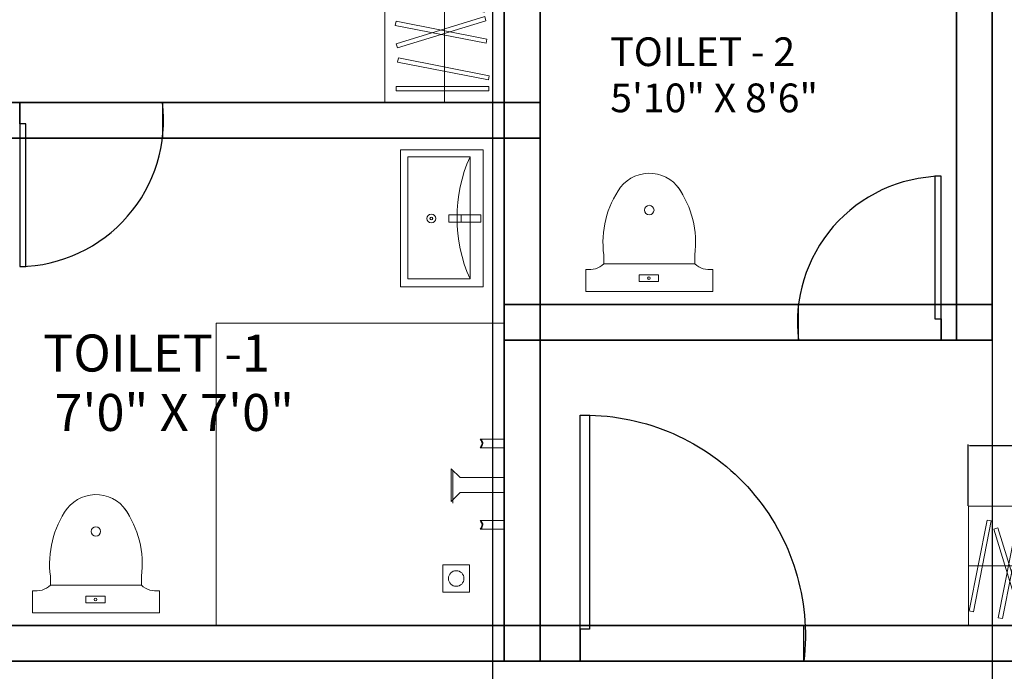
# Model space of a CAD drawing. Units: inches. Extents: x -61 to 1599, y -1316 to 257.
# Tile 67 of 204: x 240 to 406, y -790 to -680. Entities that reach past the tile are written whole.
import ezdxf

# ---------------------------------------------------------------- set-up
doc = ezdxf.new("R2010")
doc.units = ezdxf.units.IN
doc.header["$MEASUREMENT"] = 0
doc.linetypes.add('ACAD_ISO02W100', pattern=[15, 12, -3])
for name, color, linetype, lineweight in [('A-ANNO-DIMS', 2, 'Continuous', 18), ('A-AREA-IDEN', 1, 'Continuous', 18), ('A-FLOR-CASE', 8, 'Continuous', 18), ('A-FLOR-FIXT', 8, 'Continuous', 18), ('A-WALL-JAMB', 4, 'ACAD_ISO02W100', 25), ('DOORS', 2, 'Continuous', 25), ('WALLS', 4, 'Continuous', 35)]:
    doc.layers.add(name, color=color, linetype=linetype, lineweight=lineweight)
doc.styles.get("Standard").update_dxf_attribs({"font": 'arial.ttf'})
doc.dimstyles.get("Standard").update_dxf_attribs({"dimtxt": 0.18, "dimasz": 0.18, "dimexe": 0.18, "dimexo": 0.0625, "dimgap": 0.09, "dimtad": 0, "dimtih": 1, "dimtoh": 1, "dimdec": 0, "dimzin": 0, "dimdsep": 46, "dimlunit": 3, "dimtxsty": 'Standard', "dimcen": 0.09, "dimadec": 0, "dimazin": 0, "dimtfac": 1, "dimtdec": 0, "dimtofl": 0, "dimtmove": 0, "dimatfit": 3, "dimfxl": 1, "dimtolj": 1, "dimtzin": 0, "dimarcsym": 0})

# ---------------------------------------------------------------- blocks, each defined once
blk = doc.blocks.new('DOOR-SWING-24')
blk.add_line((0, 0), (0, 3.6))
blk.add_lwpolyline([(0, 0), (0, -24), (1.05, -24), (1.05, 0)], close=True)
blk.add_arc((-0.44, 0.62), 24.62, 271.0259, 6.9559)
blk = doc.blocks.new('DOOR-SWING-36')
blk.add_line((0, 0), (0, -5.4))
blk.add_lwpolyline([(0, 0), (0, 36), (-1.57, 36), (-1.57, 0)], close=True)
blk.add_arc((-0.74, -1.08), 37.09, 91.2913, 186.6905)
blk = doc.blocks.new('WC-FLOOR-MOUNT')
for p, q in [((3.02, 4.69), (3.02, 6.17)), ((18.31, 4.69), (18.31, 6.17)), ((0, 0), (0, 3.75)), ((3.02, 4.69), (18.31, 4.69)), ((21.33, 0), (21.33, 3.75)), ((0, 0), (21.33, 0))]:
    blk.add_line(p, q)
blk.add_lwpolyline([(12.24, 1.73), (8.96, 1.73), (8.96, 2.81), (12.24, 2.81)], close=True)
for centre, radius in [((10.67, 13.73), 0.792), ((10.6, 2.27), 0.208)]:
    blk.add_circle(centre, radius)
for centre, radius, start, end in [((10.67, 13.73), 6.18, 27.6844, 141.4697), ((19.05, 8.26), 16.17, 144.824, 187.4232), ((2.28, 8.26), 16.17, 352.5768, 35.176), ((0.56, 7.25), 3.55, 260.8586, 313.6993), ((20.77, 7.25), 3.55, 226.3007, 279.1414)]:
    blk.add_arc(centre, radius, start, end)
blk = doc.blocks.new('LAVATORY-WALL')
blk.add_line((10.19, 12.11), (10.19, 10.88))
for points in [[(13.87, 0), (0, 0), (0, 23.07), (13.87, 23.07)], [(13.87, 0), (0, 0), (0, 23.07), (13.87, 23.07)], [(1.2, 1.34), (1.2, 21.88), (11.67, 21.88), (11.67, 1.34)], [(8.09, 10.88), (8.09, 12.11), (13.47, 12.11), (13.47, 10.88)]]:
    blk.add_lwpolyline(points, close=True)
for radius in [0.74, 0.233]:
    blk.add_circle((5.16, 11.5), radius)
blk.add_arc((34.73, 11.61), 25.25, 155.9939, 204.0061)
blk = doc.blocks.new('SHOWER-FITTINGS')
for p, q in [((10.35, 25.72), (6.31, 25.72)), ((10.35, 24.3), (6.31, 24.3)), ((10.35, 23), (10.35, 23)), ((2.92, 19.29), (1.4, 20.76)), ((1.4, 15.27), (1.4, 20.76)), ((1.69, 14.98), (1.69, 20.48)), ((10.35, 19.29), (2.92, 19.29)), ((2.92, 16.74), (1.4, 15.27)), ((10.35, 16.74), (2.92, 16.74)), ((10.35, 12.03), (6.31, 12.03)), ((10.35, 10.61), (6.31, 10.61))]:
    blk.add_line(p, q)
blk.add_lwpolyline([(4.52, 0), (0, 0), (0, 4.57), (4.52, 4.57)], close=True)
blk.add_circle((2.26, 2.29), 1.31)
for points in [[(6.31, 24.3), (6.45, 24.53), (6.75, 25), (6.46, 25.48), (6.31, 25.72)], [(6.45, 24.3), (6.59, 24.53), (6.88, 25), (6.59, 25.48), (6.45, 25.72)], [(6.31, 10.61), (6.45, 10.84), (6.75, 11.31), (6.46, 11.78), (6.31, 12.03)], [(6.45, 10.61), (6.59, 10.84), (6.88, 11.31), (6.59, 11.78), (6.45, 12.03)]]:
    blk.add_open_spline(points, degree=3, knots=[0, 0, 0, 0, 0.7501, 1.532449, 1.532449, 1.532449, 1.532449])
blk = doc.blocks.new('WARDROBE-HANGING')
blk.add_line((10.05, 0), (10.05, 68))
for points in [[(20.09, 0), (0, 0), (0, 68), (20.09, 68)], [(2.48, 67.85), (17.75, 64.85), (17.61, 64.14), (2.34, 67.15)], [(1.32, 62.96), (16.59, 59.95), (16.45, 59.25), (1.19, 62.25)], [(1.35, 59.16), (16.22, 63.73), (16.43, 63.04), (1.56, 58.47)], [(1.71, 56.78), (16.98, 53.78), (16.84, 53.07), (1.57, 56.08)], [(1, 46.47), (15.87, 51.04), (16.08, 50.35), (1.21, 45.78)], [(1.39, 50.01), (16.66, 47.01), (16.52, 46.3), (1.26, 49.31)], [(1.36, 44.09), (16.63, 41.09), (16.49, 40.38), (1.23, 43.38)], [(1.26, 37.2), (16.53, 34.2), (16.39, 33.49), (1.12, 36.5)], [(1.28, 33.41), (16.16, 37.98), (16.37, 37.29), (1.49, 32.72)], [(1.65, 31.03), (16.92, 28.03), (16.78, 27.32), (1.51, 30.32)], [(1.26, 25.09), (16.53, 22.09), (16.39, 21.38), (1.12, 24.39)], [(1.28, 21.3), (16.15, 25.87), (16.36, 25.18), (1.49, 20.61)], [(1.65, 18.92), (16.91, 15.92), (16.78, 15.21), (1.51, 18.21)], [(1.91, 13.69), (17.17, 10.68), (17.04, 9.98), (1.77, 12.98)], [(1.93, 9.89), (16.8, 14.46), (17.01, 13.77), (2.14, 9.2)], [(2.29, 7.51), (17.56, 4.51), (17.42, 3.8), (2.16, 6.81)], [(17.49, 1.96), (1.93, 1.96), (1.93, 2.68), (17.49, 2.68)]]:
    blk.add_lwpolyline(points, close=True)
blk = doc.blocks.new('*D620')
at = {"layer": 'A-ANNO-DIMS', "color": 0, "lineweight": -2, "transparency": 16777216}
for p, q in [((399.7, -761.79), (399.7, -751.47)), ((399.88, -751.65), (432.4, -751.65)), ((467.52, -751.65), (435.01, -751.65)), ((467.7, -761.79), (467.7, -751.47))]:
    blk.add_line(p, q, dxfattribs=at)
at = {"layer": 'A-ANNO-DIMS', "color": 0, "transparency": 16777216}
for points in [[(399.88, -751.62), (399.88, -751.68), (399.7, -751.65)], [(467.52, -751.62), (467.52, -751.68), (467.7, -751.65)]]:
    blk.add_solid(points, dxfattribs=at)
at = {"layer": 'DEFPOINTS', "color": 0, "transparency": 16777216}
for p in [(399.7, -751.65), (399.7, -761.85), (467.7, -761.85)]:
    blk.add_point(p, dxfattribs=at)
at = {"layer": 'A-ANNO-DIMS', "color": 0, "transparency": 16777216, "insert": (433.7, -751.65), "char_height": 0.18, "attachment_point": 5}
blk.add_mtext('\\A1;WARDROBE 68 TYP.', dxfattribs=at)
blk = doc.blocks.new('*D687')
at = {"layer": 'A-ANNO-DIMS', "color": 0, "lineweight": -2, "transparency": 16777216}
for p, q in [((289.42, 181.68), (-61.08, 181.68)), ((-60.9, 181.5), (-60.9, -528.95)), ((-60.9, -1239.76), (-60.9, -529.32)), ((319.64, -1239.94), (-61.08, -1239.94))]:
    blk.add_line(p, q, dxfattribs=at)
at = {"layer": 'A-ANNO-DIMS', "color": 0, "transparency": 16777216}
for points in [[(-60.93, 181.5), (-60.87, 181.5), (-60.9, 181.68)], [(-60.93, -1239.76), (-60.87, -1239.76), (-60.9, -1239.94)]]:
    blk.add_solid(points, dxfattribs=at)
at = {"layer": 'DEFPOINTS', "color": 0, "transparency": 16777216}
for p in [(289.48, 181.68), (-60.9, -1239.94), (319.7, -1239.94)]:
    blk.add_point(p, dxfattribs=at)
at = {"layer": 'A-ANNO-DIMS', "color": 0, "transparency": 16777216, "insert": (-60.9, -529.13), "char_height": 0.18, "attachment_point": 5}
blk.add_mtext('\\A1;1421.6', dxfattribs=at)
blk = doc.blocks.new('*D710')
at = {"layer": 'A-ANNO-DIMS', "color": 0, "lineweight": -2, "transparency": 16777216}
for p, q in [((319.7, -465.39), (319.7, -1315.72)), ((403.7, -465.39), (403.7, -1315.72)), ((319.88, -1315.54), (361.48, -1315.54)), ((403.52, -1315.54), (361.92, -1315.54))]:
    blk.add_line(p, q, dxfattribs=at)
at = {"layer": 'A-ANNO-DIMS', "color": 0, "transparency": 16777216}
for points in [[(319.88, -1315.51), (319.88, -1315.57), (319.7, -1315.54)], [(403.52, -1315.51), (403.52, -1315.57), (403.7, -1315.54)]]:
    blk.add_solid(points, dxfattribs=at)
at = {"layer": 'DEFPOINTS', "color": 0, "transparency": 16777216}
for p in [(319.7, -465.32), (403.7, -465.32), (403.7, -1315.54)]:
    blk.add_point(p, dxfattribs=at)
at = {"layer": 'A-ANNO-DIMS', "color": 0, "transparency": 16777216, "insert": (361.7, -1315.54), "char_height": 0.18, "attachment_point": 5}
blk.add_mtext('\\A1;84', dxfattribs=at)

msp = doc.modelspace()

# ---------------------------------------------------------------- linework, layer by layer
at = {"layer": 'A-FLOR-FIXT'}
for p, q in [((321.7028, -731.0902), (273.2827, -731.0902)), ((273.2827, -731.0902), (273.2827, -781.9446))]:
    msp.add_line(p, q, dxfattribs=at)
at = {"layer": 'A-WALL-JAMB'}
for p, q in [((240.2351, -693.9446), (240.2351, -699.9446)), ((264.2351, -693.9446), (264.2306, -699.9446)), ((371.1461, -733.9446), (371.1461, -727.9446)), ((395.1461, -733.9446), (395.1461, -727.9446)), ((334.4752, -787.9446), (334.4752, -781.9446)), ((372.0502, -787.9446), (372.0502, -781.9446))]:
    msp.add_line(p, q, dxfattribs=at)
at = {"layer": 'WALLS'}
for p, q in [((321.7028, -616.9446), (321.7028, -787.9446)), ((327.7028, -616.9446), (327.7028, -787.9446)), ((397.7028, -616.9446), (397.7028, -733.9446)), ((403.7028, -616.9446), (403.7028, -733.9446)), ((231.7028, -693.9446), (327.7028, -693.9446)), ((231.7028, -699.9446), (327.7028, -699.9446)), ((321.7028, -727.9446), (403.7028, -727.9446)), ((321.7028, -733.9446), (403.7028, -733.9446)), ((237.7028, -781.9446), (327.7028, -781.9446)), ((321.7028, -781.9446), (403.7028, -781.9446)), ((397.7028, -781.9446), (535.7028, -781.9446)), ((237.7028, -787.9446), (327.7028, -787.9446)), ((321.7028, -787.9446), (403.7028, -787.9446)), ((397.7028, -787.9446), (535.7028, -787.9446))]:
    msp.add_line(p, q, dxfattribs=at)

# ---------------------------------------------------------------- block references
at = {"layer": 'A-FLOR-CASE'}
msp.add_blockref('WARDROBE-HANGING', (301.609, -693.9447), dxfattribs=at)
at = {"layer": 'A-FLOR-CASE', "rotation": 90.00000000000078}
msp.add_blockref('WARDROBE-HANGING', (467.7029, -781.9448), dxfattribs=at)
at = {"layer": 'A-FLOR-FIXT'}
for name, p in [('LAVATORY-WALL', (304.2705, -724.9583)), ('WC-FLOOR-MOUNT', (335.402, -725.7577)), ('SHOWER-FITTINGS', (311.351, -776.3107)), ('WC-FLOOR-MOUNT', (242.3826, -779.8229))]:
    msp.add_blockref(name, p, dxfattribs=at)
at = {"layer": 'DOORS'}
msp.add_blockref('DOOR-SWING-24', (240.2351, -697.5446), dxfattribs=at)
at = {"layer": 'DOORS', "rotation": 180}
msp.add_blockref('DOOR-SWING-24', (395.1461, -730.3446), dxfattribs=at)
at = {"layer": 'DOORS', "extrusion": (0, 0, -1), "zscale": -1}
msp.add_blockref('DOOR-SWING-36', (-334.4752, -782.5446), dxfattribs=at)

# ---------------------------------------------------------------- texts
at = {"layer": 'A-AREA-IDEN'}
for s, height, p in [('TOILET - 2', 4.8321, (339.5043, -687.8122)), ('5\'10" X 8\'6"', 4.832098, (339.5043, -695.5745)), (' TOILET -1', 6.22364, (242.2634, -739.1989)), ('  7\'0" X 7\'0"', 6.223643, (242.2634, -749.1966))]:
    msp.add_text(s, height=height, dxfattribs=at).set_placement(p)

# ---------------------------------------------------------------- dimensions: what is measured, and where the dimension line sits
at = {"layer": 'A-ANNO-DIMS'}
dim = msp.add_linear_dim(base=(-60.8972, -1239.9446), p1=(289.4807, 181.6771), p2=(319.7028, -1239.9446), angle=90, dimstyle='Standard', override={"dimdec": 1, "dimlfac": 1, "dimrnd": 0, "dimzin": 0, "dimdsep": 46, "dimlunit": 2}, dxfattribs=at)
dim.commit()
dim.dimension.update_dxf_attribs({"geometry": '*D687', "text_midpoint": (-60.8972, -529.1337)})
dim = msp.add_linear_dim(base=(403.7028, -1315.5446), p1=(319.7028, -465.3229), p2=(403.7028, -465.3229), dimstyle='Standard', override={"dimdec": 0, "dimlfac": 1, "dimrnd": 0, "dimzin": 0, "dimdsep": 46, "dimlunit": 2}, dxfattribs=at)
dim.commit()
dim.dimension.update_dxf_attribs({"geometry": '*D710', "text_midpoint": (361.7028, -1315.5446)})
dim = msp.add_linear_dim(base=(399.7028, -751.651), p1=(467.7028, -761.851), p2=(399.7028, -761.851), angle=180, text='WARDROBE <> TYP.', dimstyle='Standard', override={"dimdec": 0, "dimlfac": 1, "dimrnd": 0, "dimzin": 0, "dimdsep": 46, "dimlunit": 2}, dxfattribs=at)
dim.commit()
dim.dimension.update_dxf_attribs({"geometry": '*D620', "text_midpoint": (433.7028, -751.651)})

doc.saveas('drawing.dxf')
